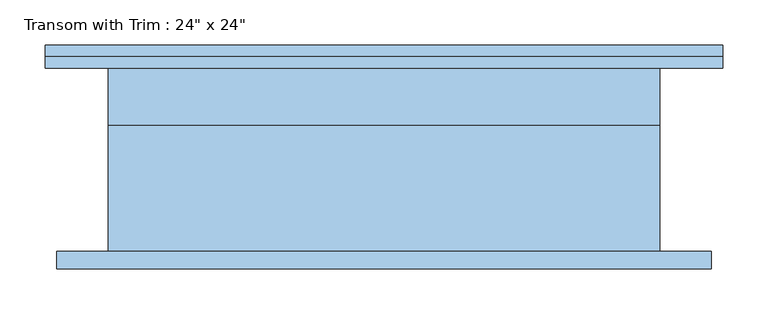
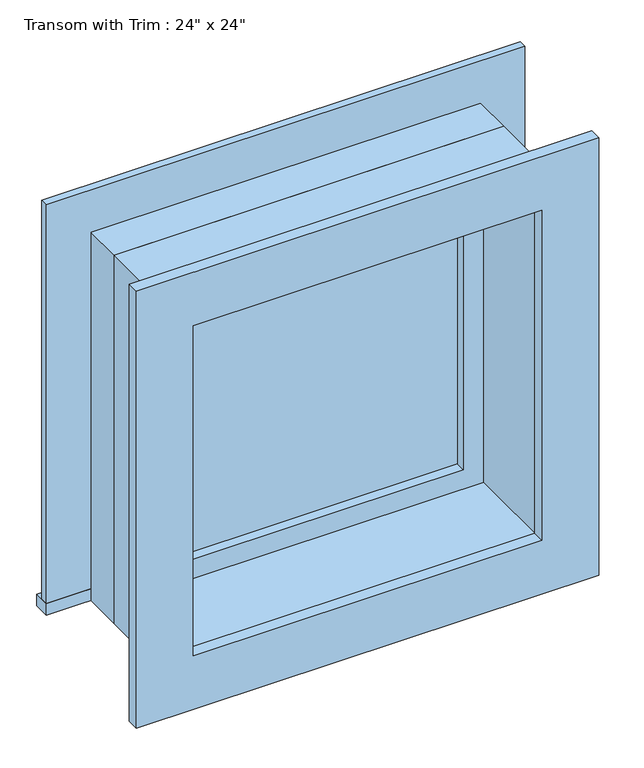
"""IFC4 building model written with IfcOpenShell, lengths in millimetres: window geometry."""

from ifc_helpers import new_model, si_unit, frame, origin, place, context, project, spatial, polyline, outline, extrude, source, transform, mapped, element, save


def window_e41d21a6(model_context):
    return source(origin(), model_context, "Body", "SweptSolid", [
        extrude(outline(polyline([(-412.75, 127.0), (336.55, 127.0), (336.55, 101.6), (-412.75, 101.6), (-412.75, 127.0)])), frame((0.0, 0.0, 2159.0), z_axis=(0.0, 0.0, 1.0), x_axis=(1.0, 0.0, 0.0)), (0.0, 0.0, 1.0), 19.05),
        extrude(outline(polyline([(2749.55, -323.85), (2749.55, 247.65), (2178.05, 247.65), (2178.05, 336.55), (2838.45, 336.55), (2838.45, -412.75), (2178.05, -412.75), (2178.05, -323.85), (2749.55, -323.85)])), frame((0.0, 101.6, 0.0), z_axis=(0.0, 1.0, 0.0), x_axis=(0.0, 0.0, 1.0)), (0.0, 0.0, 1.0), 12.7),
        extrude(outline(polyline([(2825.75, 323.85), (2825.75, -400.05), (2101.85, -400.05), (2101.85, 323.85), (2825.75, 323.85)]), holes=[polyline([(2736.85, 234.95), (2190.75, 234.95), (2190.75, -311.15), (2736.85, -311.15), (2736.85, 234.95)])]), frame((0.0, -120.65, 0.0), z_axis=(0.0, 1.0, 0.0), x_axis=(0.0, 0.0, 1.0)), (0.0, 0.0, 1.0), 19.05),
        extrude(outline(polyline([(203.2, 53.975), (-279.4, 53.975), (-279.4, 66.675), (203.2, 66.675), (203.2, 53.975)])), frame((0.0, 0.0, 2222.5), z_axis=(0.0, 0.0, 1.0), x_axis=(1.0, 0.0, 0.0)), (0.0, 0.0, 1.0), 482.6),
        extrude(outline(polyline([(2749.55, -323.85), (2178.05, -323.85), (2178.05, 247.65), (2749.55, 247.65), (2749.55, -323.85)]), holes=[polyline([(2705.1, -279.4), (2705.1, 203.2), (2222.5, 203.2), (2222.5, -279.4), (2705.1, -279.4)])]), frame((0.0, 38.1, 0.0), z_axis=(0.0, 1.0, 0.0), x_axis=(0.0, 0.0, 1.0)), (0.0, 0.0, 1.0), 44.45),
        extrude(outline(polyline([(2768.6, -342.9), (2159.0, -342.9), (2159.0, 266.7), (2768.6, 266.7), (2768.6, -342.9)]), holes=[polyline([(2736.85, -311.15), (2736.85, 234.95), (2190.75, 234.95), (2190.75, -311.15), (2736.85, -311.15)])]), frame((0.0, -101.6, 0.0), z_axis=(0.0, 1.0, 0.0), x_axis=(0.0, 0.0, 1.0)), (0.0, 0.0, 1.0), 139.7),
        extrude(outline(polyline([(2768.6, 266.7), (2768.6, -342.9), (2159.0, -342.9), (2159.0, 266.7), (2768.6, 266.7)]), holes=[polyline([(2749.55, 247.65), (2178.05, 247.65), (2178.05, -323.85), (2749.55, -323.85), (2749.55, 247.65)])]), frame((0.0, 38.1, 0.0), z_axis=(0.0, 1.0, 0.0), x_axis=(0.0, 0.0, 1.0)), (0.0, 0.0, 1.0), 63.5),
    ])


if __name__ == "__main__":
    model = new_model("IFC4")
    model_context = context("Model", 3, world=origin())
    ifc_project = project(units=[si_unit("LENGTHUNIT", "METRE", prefix="MILLI")], contexts=[model_context])
    site = spatial("IfcSite", under=ifc_project)
    building = spatial("IfcBuilding", under=site)
    placement = place(None, origin())
    window_shape = window_e41d21a6(model_context)
    element("IfcWindow", 1, ObjectType="Transom with Trim : 24\" x 24\"", at=placement, inside=building, context=model_context, shape_type="MappedRepresentation", body=[
        mapped(window_shape, transform((0.0, 0.0, 0.0), x_axis=(1.0, 0.0, 0.0), y_axis=(0.0, 1.0, 0.0), z_axis=(0.0, 0.0, 1.0))),
    ])
    save(model, "model.ifc")

# Revit data of these elements
# Type "Transom with Trim : 24\" x 24\""
#   Type Mark = "10"
#   Construction Type Id = "GSP4R"
#   Assembly Code = "B2020100"
#   Analytic Construction = "1/8 in Pilkington single glazing"
#   Visual Light Transmittance = 0.9
#   Solar Heat Gain Coefficient = 0.78
#   Heat Transfer Coefficient (U) = 0.6496 BTU/(h·ft²·°F)
#   Height = 2' - 0"
#   Default Sill Height = 7' - 1"
#   Trim Projection - Ext. = 0' - 0 1/2"
#   Trim Projection - Int. = 0' - 0 3/4"
#   Trim Width - Exterior = 0' - 3 1/2"
#   Trim Width - Interior = 0' - 3 1/2"
#   Width = 2' - 0"
#   Window Inset = 0' - 0 3/4"
#   Define Thermal Properties by = 1
#   Glass Pane Material = Glass
#   Sash Material = Sash
#   Trim Exterior Material = Trim
#   Trim Interior Material = Trim
#   Wall Closure = (empty or 0)
# Element 1 (IfcWindow, "Transom with Trim : 24\" x 24\"")
#   Materials on its faces: "Sash", "Trim", "Glass"
# Materials
#   "Glass": class "Glass", colour RGB 0 128 192, transparency 0.75, Description = "Soda Lime Glass", Cost = 0
#   "Sash": class "Wood", colour RGB 224 178 126, transparency 0
#   "Trim": class "Wood", colour RGB 224 178 126, transparency 0
